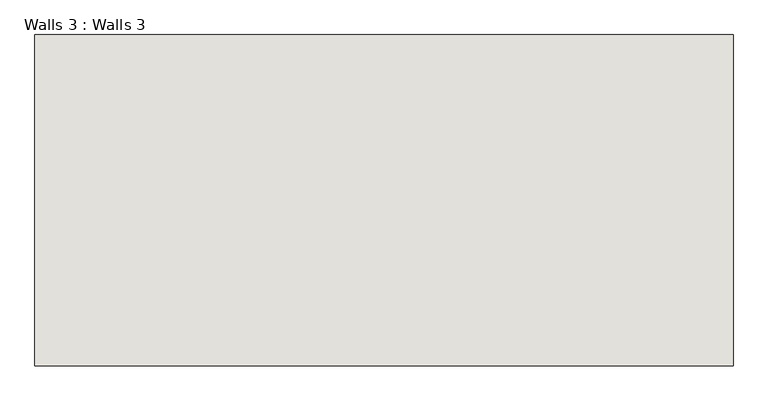
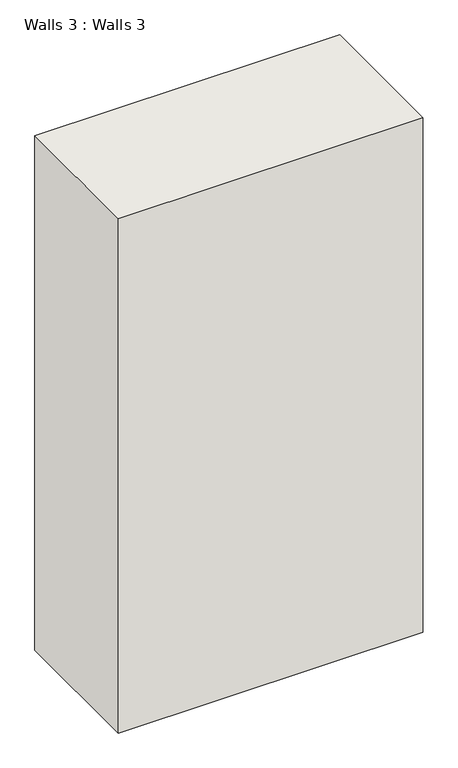
"""IFC4 building model written with IfcOpenShell, lengths in millimetres: wall geometry, Walls 3 : Walls 3."""

from ifc_helpers import new_model, si_unit, origin, origin_with_axes, place, context, project, spatial, polyline, outline, extrude, source, transform, mapped, element, save


def walls_3_walls_3_385398a2(model_context):
    return source(origin(), model_context, "Body", "SweptSolid", [
        extrude(outline(polyline([(-1020.9821198, 1301.80098), (-2642.9841378, 1301.80098), (-2642.9841378, 2071.2670553), (-1020.9821198, 2071.2670553), (-1020.9821198, 1301.80098)])), origin_with_axes(), (0.0, 0.0, 1.0), 2895.6),
    ])


if __name__ == "__main__":
    model = new_model("IFC4")
    model_context = context("Model", 3, world=origin())
    ifc_project = project(units=[si_unit("LENGTHUNIT", "METRE", prefix="MILLI")], contexts=[model_context])
    site = spatial("IfcSite", under=ifc_project)
    building = spatial("IfcBuilding", under=site)
    placement = place(None, origin())
    walls_3_walls_3_shape = walls_3_walls_3_385398a2(model_context)
    element("IfcWall", 1, ObjectType="Walls 3 : Walls 3", at=placement, inside=building, context=model_context, shape_type="MappedRepresentation", body=[
        mapped(walls_3_walls_3_shape, transform((0.0, 0.0, 0.0), x_axis=(1.0, 0.0, 0.0), y_axis=(0.0, 1.0, 0.0), z_axis=(0.0, 0.0, 1.0))),
    ])
    save(model, "model.ifc")

# Revit data of these elements
# Element 1 (IfcWall, "Walls 3 : Walls 3")
#   Materials on its faces: "Default Wall"
# Materials
#   "Default Wall": colour RGB 128 128 128, transparency 0
